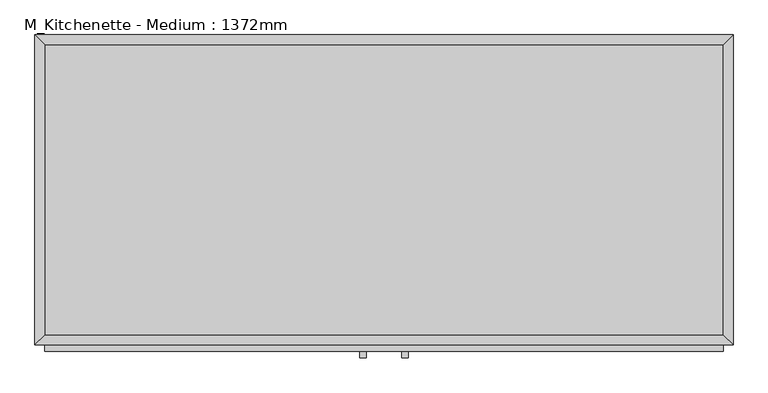
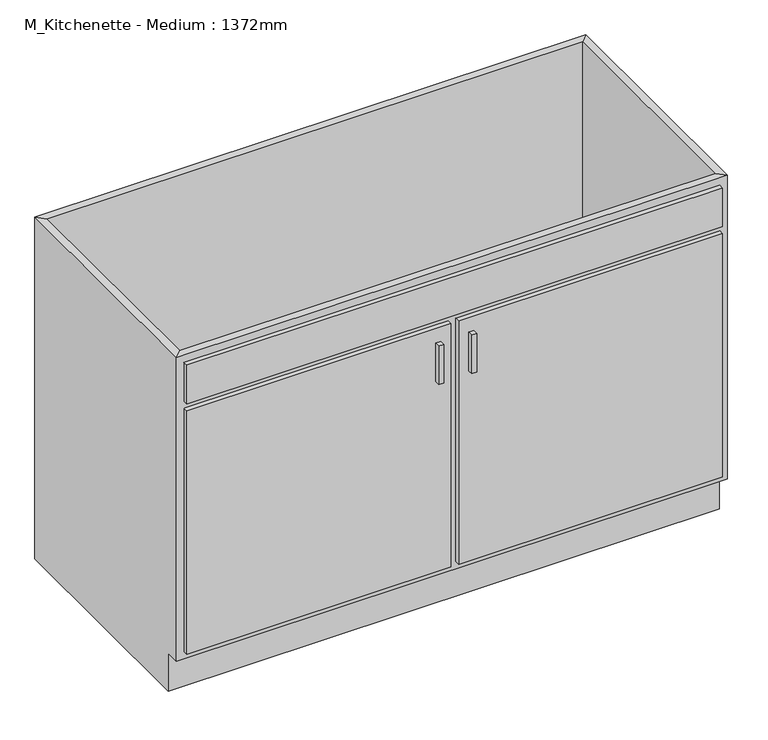
"""IFC4 building model written with IfcOpenShell, lengths in millimetres: proxy geometry, M_Kitchenette - Medium : 1372mm."""

from ifc_helpers import new_model, si_unit, frame, origin, place, context, project, spatial, polyline, outline, extrude, faceted_brep, source, transform, mapped, element, save


def m_kitchenette_medium_1372mm_e05c6bec(model_context):
    return source(origin(), model_context, "Body", "SolidModel", [
        faceted_brep([(685.6877049, -590.95, 900.0), (685.6877049, -590.95, 100.0), (-648.2122951, -590.95, 100.0), (-648.2122951, -590.95, 900.0), (-667.2622951, -610.0, 900.0), (704.7377049, -610.0, 900.0), (-667.2622951, -610.0, 100.0), (704.7377049, -610.0, 100.0), (-648.2122951, -575.0, 100.0), (-648.2122951, -19.05, 100.0), (-648.2122951, -19.05, 900.0), (-667.2622951, 0.0, 900.0), (-667.2622951, 0.0, 0.0), (-667.2622951, -575.0, 0.0), (-667.2622951, -575.0, 100.0), (685.6877049, -19.05, 100.0), (685.6877049, -19.05, 900.0), (704.7377049, 0.0, 900.0), (704.7377049, 0.0, 0.0), (685.6877049, -575.0, 100.0), (704.7377049, -575.0, 100.0), (704.7377049, -575.0, 0.0)], [[[0, 1, 2, 3]], [[0, 3, 4, 5]], [[5, 4, 6, 7]], [[2, 1, 7, 6]], [[3, 2, 8, 9, 10]], [[4, 3, 10, 11]], [[6, 4, 11, 12, 13, 14]], [[2, 6, 14, 8]], [[10, 9, 15, 16]], [[11, 10, 16, 17]], [[12, 11, 17, 18]], [[1, 0, 16, 15, 19]], [[0, 5, 17, 16]], [[5, 7, 20, 21, 18, 17]], [[7, 1, 19, 20]], [[8, 19, 15, 9]], [[18, 21, 13, 12]], [[13, 21, 20, 19, 8, 14]]]),
        extrude(outline(polyline([(-16.1872951, -635.4), (-28.8872951, -635.4), (-28.8872951, -622.7), (-16.1872951, -622.7), (-16.1872951, -635.4)])), frame((0.0, 0.0, 620.6), z_axis=(0.0, 0.0, 1.0), x_axis=(1.0, 0.0, 0.0)), (0.0, 0.0, 1.0), 101.6),
        extrude(outline(polyline([(66.3627049, -635.4), (53.6627049, -635.4), (53.6627049, -622.7), (66.3627049, -622.7), (66.3627049, -635.4)])), frame((0.0, 0.0, 620.6), z_axis=(0.0, 0.0, 1.0), x_axis=(1.0, 0.0, 0.0)), (0.0, 0.0, 1.0), 101.6),
        extrude(outline(polyline([(685.6877049, -19.05), (685.6877049, -590.95), (-648.2122951, -590.95), (-648.2122951, -19.05), (685.6877049, -19.05)])), frame((0.0, 0.0, 100.0), z_axis=(0.0, 0.0, 1.0), x_axis=(1.0, 0.0, 0.0)), (0.0, 0.0, 1.0), 19.05),
        extrude(outline(polyline([(9.2127049, -622.7), (-648.2122951, -622.7), (-648.2122951, -610.0), (9.2127049, -610.0), (9.2127049, -622.7)])), frame((0.0, 0.0, 119.05), z_axis=(0.0, 0.0, 1.0), x_axis=(1.0, 0.0, 0.0)), (0.0, 0.0, 1.0), 641.25),
        extrude(outline(polyline([(685.6877049, -622.7), (28.2627049, -622.7), (28.2627049, -610.0), (685.6877049, -610.0), (685.6877049, -622.7)])), frame((0.0, 0.0, 119.05), z_axis=(0.0, 0.0, 1.0), x_axis=(1.0, 0.0, 0.0)), (0.0, 0.0, 1.0), 641.25),
        extrude(outline(polyline([(685.6877049, -622.7), (-648.2122951, -622.7), (-648.2122951, -610.0), (685.6877049, -610.0), (685.6877049, -622.7)])), frame((0.0, 0.0, 779.35), z_axis=(0.0, 0.0, 1.0), x_axis=(1.0, 0.0, 0.0)), (0.0, 0.0, 1.0), 101.6),
    ])


if __name__ == "__main__":
    model = new_model("IFC4")
    model_context = context("Model", 3, world=origin())
    ifc_project = project(units=[si_unit("LENGTHUNIT", "METRE", prefix="MILLI")], contexts=[model_context])
    site = spatial("IfcSite", under=ifc_project)
    building = spatial("IfcBuilding", under=site)
    placement = place(None, origin())
    m_kitchenette_medium_1372mm_shape = m_kitchenette_medium_1372mm_e05c6bec(model_context)
    element("IfcBuildingElementProxy", 1, Name="M_Kitchenette - Medium : 1372mm", ObjectType="M_Kitchenette - Medium : 1372mm", at=placement, inside=building, context=model_context, shape_type="MappedRepresentation", body=[
        mapped(m_kitchenette_medium_1372mm_shape, transform((0.0, 0.0, 0.0), x_axis=(1.0, 0.0, 0.0), y_axis=(0.0, 1.0, 0.0), z_axis=(0.0, 0.0, 1.0))),
    ])
    save(model, "model.ifc")

# Revit data of these elements
# Type "M_Kitchenette - Medium : 1372mm"
#   Counter Length = 6' - 5.95276"
#   Cabinet Width = 4' - 6.01575"
#   Cabinet Height = 2' - 11.43307"
#   Cabinet Depth = 2' - 0.01575"
#   Toe Depth = 0' - 1.37795"
#   Toe Height = 0' - 3.93701"
#   Cabinet Material = Cabinets
#   Door/Drawer Material = Cabinets
#   Handle Material = Cabinets - Handles
#   Default Elevation = 0
# Element 1 (IfcBuildingElementProxy, "M_Kitchenette - Medium : 1372mm")
#   Materials on its faces: "Cabinets", "Cabinets - Handles"
# Materials
#   "Cabinets": colour RGB 249 249 249, transparency 0
#   "Cabinets - Handles": class "Metal", colour RGB 57 57 57, transparency 0
